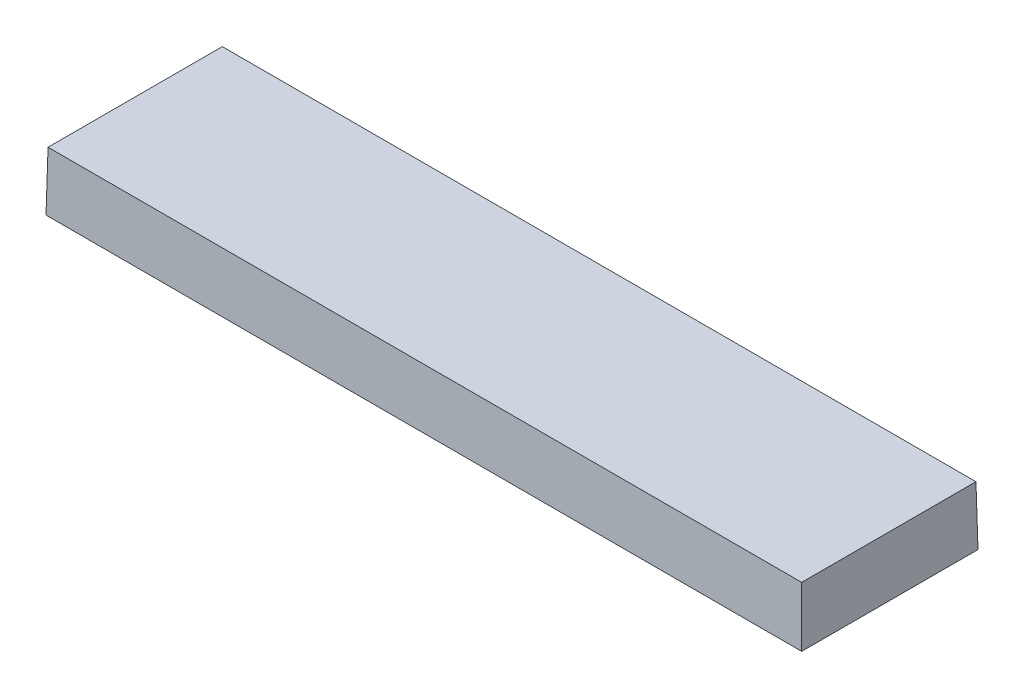
ISO-10303-21;
HEADER;
FILE_DESCRIPTION(('STEP AP214'),'2;1');
FILE_NAME('part.step','',(''),(''),'','','');
FILE_SCHEMA(('AUTOMOTIVE_DESIGN { 1 0 10303 214 1 1 1 1 }'));
ENDSEC;
DATA;
#1=APPLICATION_CONTEXT('core data for automotive mechanical design processes');
#2=APPLICATION_PROTOCOL_DEFINITION('international standard','automotive_design',2000,#1);
#3=PRODUCT_CONTEXT('',#1,'mechanical');
#4=PRODUCT('Part','Part','',(#3));
#5=PRODUCT_RELATED_PRODUCT_CATEGORY('part','',(#4));
#6=PRODUCT_DEFINITION_FORMATION('','',#4);
#7=PRODUCT_DEFINITION_CONTEXT('part definition',#1,'design');
#8=PRODUCT_DEFINITION('design','',#6,#7);
#9=PRODUCT_DEFINITION_SHAPE('','',#8);
#10=(LENGTH_UNIT() NAMED_UNIT(*) SI_UNIT(.MILLI.,.METRE.));
#11=(NAMED_UNIT(*) PLANE_ANGLE_UNIT() SI_UNIT($,.RADIAN.));
#12=(NAMED_UNIT(*) SI_UNIT($,.STERADIAN.) SOLID_ANGLE_UNIT());
#13=UNCERTAINTY_MEASURE_WITH_UNIT(LENGTH_MEASURE(1.E-05),#10,'distance_accuracy_value','');
#14=(GEOMETRIC_REPRESENTATION_CONTEXT(3) GLOBAL_UNCERTAINTY_ASSIGNED_CONTEXT((#13)) GLOBAL_UNIT_ASSIGNED_CONTEXT((#10,
#11,#12)) REPRESENTATION_CONTEXT('',''));
#15=CARTESIAN_POINT('',(0.,0.,0.));
#16=DIRECTION('',(0.,0.,1.));
#17=DIRECTION('',(1.,0.,0.));
#18=AXIS2_PLACEMENT_3D('',#15,#16,#17);
#19=CARTESIAN_POINT('',(45.,0.,-10.5));
#20=DIRECTION('',(0.999847695156391,0.0174524064372835,0.));
#21=DIRECTION('',(-0.0174524064372836,0.999847695156391,0.));
#22=AXIS2_PLACEMENT_3D('',#19,#20,#21);
#23=PLANE('',#22);
#24=DIRECTION('',(0.,0.,-1.));
#25=VECTOR('',#24,1.);
#26=CARTESIAN_POINT('',(45.,0.,-10.5));
#27=LINE('',#26,#25);
#28=CARTESIAN_POINT('',(45.,0.,10.5));
#29=VERTEX_POINT('',#28);
#30=CARTESIAN_POINT('',(45.,0.,-10.5));
#31=VERTEX_POINT('',#30);
#32=EDGE_CURVE('E85',#29,#31,#27,.T.);
#33=ORIENTED_EDGE('',*,*,#32,.T.);
#34=DIRECTION('',(0.0174497491606827,-0.999695459881887,-0.0174497491606827));
#35=VECTOR('',#34,1.);
#36=CARTESIAN_POINT('',(44.9725955628806,1.56999915108111,-10.4725955628806));
#37=LINE('',#36,#35);
#38=CARTESIAN_POINT('',(44.8778145455025,7.,-10.3778145455025));
#39=VERTEX_POINT('',#38);
#40=EDGE_CURVE('E11',#39,#31,#37,.T.);
#41=ORIENTED_EDGE('',*,*,#40,.F.);
#42=DIRECTION('',(0.,0.,1.));
#43=VECTOR('',#42,1.);
#44=CARTESIAN_POINT('',(44.8778145455025,7.,-10.5));
#45=LINE('',#44,#43);
#46=CARTESIAN_POINT('',(44.8778145455025,7.,10.3778145455025));
#47=VERTEX_POINT('',#46);
#48=EDGE_CURVE('E101',#47,#39,#45,.F.);
#49=ORIENTED_EDGE('',*,*,#48,.F.);
#50=DIRECTION('',(0.0174497491606827,-0.999695459881887,0.0174497491606827));
#51=VECTOR('',#50,1.);
#52=CARTESIAN_POINT('',(44.9936056313388,0.366333135252258,10.4936056313388));
#53=LINE('',#52,#51);
#54=EDGE_CURVE('E96',#47,#29,#53,.T.);
#55=ORIENTED_EDGE('',*,*,#54,.T.);
#56=EDGE_LOOP('',(#33,#41,#49,#55));
#57=FACE_BOUND('',#56,.T.);
#58=ADVANCED_FACE('F39',(#57),#23,.T.);
#59=CARTESIAN_POINT('',(-45.,0.,-10.5));
#60=DIRECTION('',(0.,0.0174524064372835,-0.999847695156391));
#61=DIRECTION('',(0.,0.999847695156391,0.0174524064372836));
#62=AXIS2_PLACEMENT_3D('',#59,#60,#61);
#63=PLANE('',#62);
#64=DIRECTION('',(-1.,0.,0.));
#65=VECTOR('',#64,1.);
#66=CARTESIAN_POINT('',(-45.,0.,-10.5));
#67=LINE('',#66,#65);
#68=CARTESIAN_POINT('',(-45.,0.,-10.5));
#69=VERTEX_POINT('',#68);
#70=EDGE_CURVE('E81',#31,#69,#67,.T.);
#71=ORIENTED_EDGE('',*,*,#70,.T.);
#72=DIRECTION('',(-0.0174497491606827,-0.999695459881887,-0.0174497491606827));
#73=VECTOR('',#72,1.);
#74=CARTESIAN_POINT('',(-45.,0.,-10.5));
#75=LINE('',#74,#73);
#76=CARTESIAN_POINT('',(-44.8778145455025,7.,-10.3778145455025));
#77=VERTEX_POINT('',#76);
#78=EDGE_CURVE('E48',#77,#69,#75,.T.);
#79=ORIENTED_EDGE('',*,*,#78,.F.);
#80=DIRECTION('',(1.,0.,0.));
#81=VECTOR('',#80,1.);
#82=CARTESIAN_POINT('',(-45.,7.,-10.3778145455025));
#83=LINE('',#82,#81);
#84=EDGE_CURVE('E95',#39,#77,#83,.F.);
#85=ORIENTED_EDGE('',*,*,#84,.F.);
#86=ORIENTED_EDGE('',*,*,#40,.T.);
#87=EDGE_LOOP('',(#71,#79,#85,#86));
#88=FACE_BOUND('',#87,.T.);
#89=ADVANCED_FACE('F41',(#88),#63,.T.);
#90=CARTESIAN_POINT('',(-45.,0.,-10.5));
#91=DIRECTION('',(-0.999847695156391,0.0174524064372835,0.));
#92=DIRECTION('',(-0.0174524064372836,-0.999847695156391,0.));
#93=AXIS2_PLACEMENT_3D('',#90,#91,#92);
#94=PLANE('',#93);
#95=DIRECTION('',(0.,0.,1.));
#96=VECTOR('',#95,1.);
#97=CARTESIAN_POINT('',(-45.,0.,-10.5));
#98=LINE('',#97,#96);
#99=CARTESIAN_POINT('',(-45.,0.,10.5));
#100=VERTEX_POINT('',#99);
#101=EDGE_CURVE('E88',#69,#100,#98,.T.);
#102=ORIENTED_EDGE('',*,*,#101,.T.);
#103=DIRECTION('',(-0.0174497491606827,-0.999695459881887,0.0174497491606827));
#104=VECTOR('',#103,1.);
#105=CARTESIAN_POINT('',(-45.,0.,10.5));
#106=LINE('',#105,#104);
#107=CARTESIAN_POINT('',(-44.8778145455025,7.,10.3778145455025));
#108=VERTEX_POINT('',#107);
#109=EDGE_CURVE('E102',#108,#100,#106,.T.);
#110=ORIENTED_EDGE('',*,*,#109,.F.);
#111=DIRECTION('',(0.,0.,-1.));
#112=VECTOR('',#111,1.);
#113=CARTESIAN_POINT('',(-44.8778145455025,7.,-10.5));
#114=LINE('',#113,#112);
#115=EDGE_CURVE('E58',#77,#108,#114,.F.);
#116=ORIENTED_EDGE('',*,*,#115,.F.);
#117=ORIENTED_EDGE('',*,*,#78,.T.);
#118=EDGE_LOOP('',(#102,#110,#116,#117));
#119=FACE_BOUND('',#118,.T.);
#120=ADVANCED_FACE('F112',(#119),#94,.T.);
#121=CARTESIAN_POINT('',(-45.,0.,10.5));
#122=DIRECTION('',(0.,0.0174524064372835,0.999847695156391));
#123=DIRECTION('',(0.,-0.999847695156391,0.0174524064372836));
#124=AXIS2_PLACEMENT_3D('',#121,#122,#123);
#125=PLANE('',#124);
#126=DIRECTION('',(1.,0.,0.));
#127=VECTOR('',#126,1.);
#128=CARTESIAN_POINT('',(-45.,0.,10.5));
#129=LINE('',#128,#127);
#130=EDGE_CURVE('E99',#100,#29,#129,.T.);
#131=ORIENTED_EDGE('',*,*,#130,.T.);
#132=ORIENTED_EDGE('',*,*,#54,.F.);
#133=DIRECTION('',(-1.,0.,0.));
#134=VECTOR('',#133,1.);
#135=CARTESIAN_POINT('',(-45.,7.,10.3778145455025));
#136=LINE('',#135,#134);
#137=EDGE_CURVE('E43',#108,#47,#136,.F.);
#138=ORIENTED_EDGE('',*,*,#137,.F.);
#139=ORIENTED_EDGE('',*,*,#109,.T.);
#140=EDGE_LOOP('',(#131,#132,#138,#139));
#141=FACE_BOUND('',#140,.T.);
#142=ADVANCED_FACE('F114',(#141),#125,.T.);
#143=CARTESIAN_POINT('',(0.,7.,0.));
#144=DIRECTION('',(0.,1.,0.));
#145=DIRECTION('',(0.,0.,1.));
#146=AXIS2_PLACEMENT_3D('',#143,#144,#145);
#147=PLANE('',#146);
#148=ORIENTED_EDGE('',*,*,#48,.T.);
#149=ORIENTED_EDGE('',*,*,#84,.T.);
#150=ORIENTED_EDGE('',*,*,#115,.T.);
#151=ORIENTED_EDGE('',*,*,#137,.T.);
#152=EDGE_LOOP('',(#148,#149,#150,#151));
#153=FACE_BOUND('',#152,.T.);
#154=ADVANCED_FACE('F108',(#153),#147,.T.);
#155=CARTESIAN_POINT('',(0.,0.,0.));
#156=DIRECTION('',(0.,1.,0.));
#157=DIRECTION('',(0.,0.,1.));
#158=AXIS2_PLACEMENT_3D('',#155,#156,#157);
#159=PLANE('',#158);
#160=ORIENTED_EDGE('',*,*,#32,.F.);
#161=ORIENTED_EDGE('',*,*,#130,.F.);
#162=ORIENTED_EDGE('',*,*,#101,.F.);
#163=ORIENTED_EDGE('',*,*,#70,.F.);
#164=EDGE_LOOP('',(#160,#161,#162,#163));
#165=FACE_BOUND('',#164,.T.);
#166=ADVANCED_FACE('F82',(#165),#159,.F.);
#167=CLOSED_SHELL('',(#58,#89,#120,#142,#154,#166));
#168=MANIFOLD_SOLID_BREP('B2',#167);
#169=ADVANCED_BREP_SHAPE_REPRESENTATION('',(#18,#168),#14);
#170=SHAPE_DEFINITION_REPRESENTATION(#9,#169);
ENDSEC;
END-ISO-10303-21;
